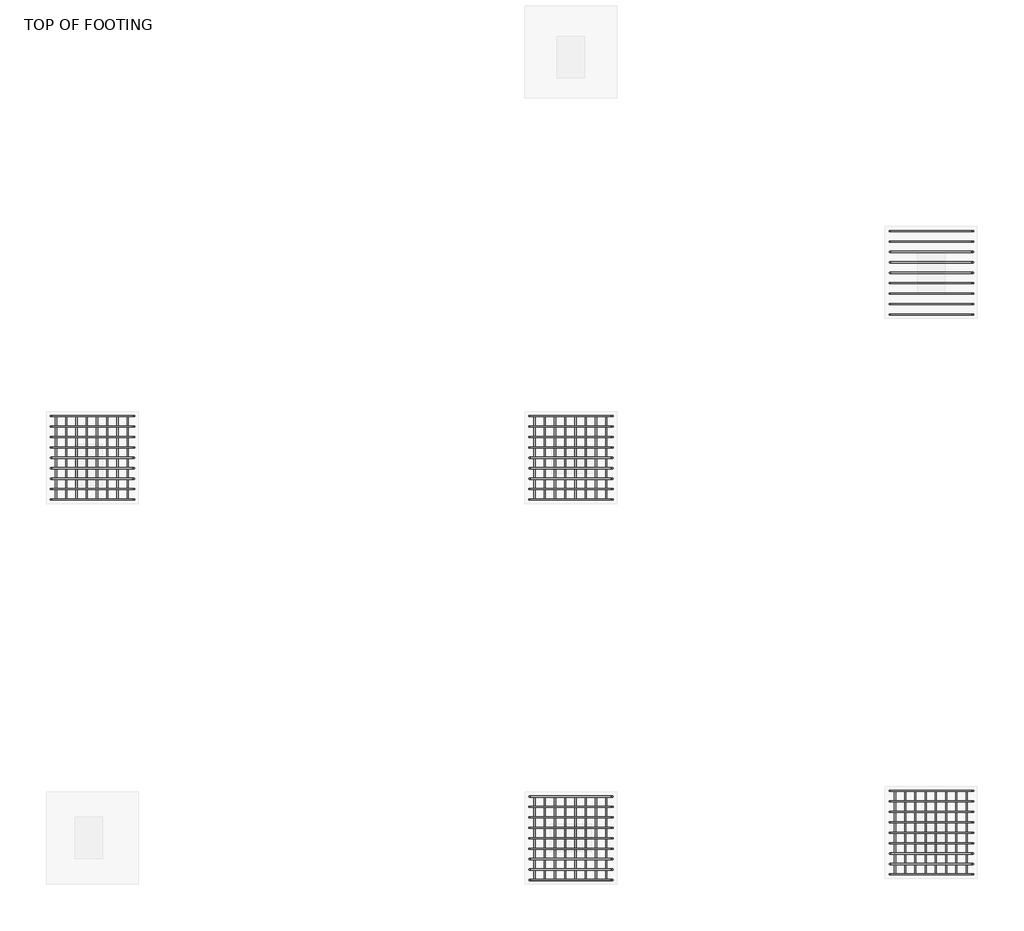
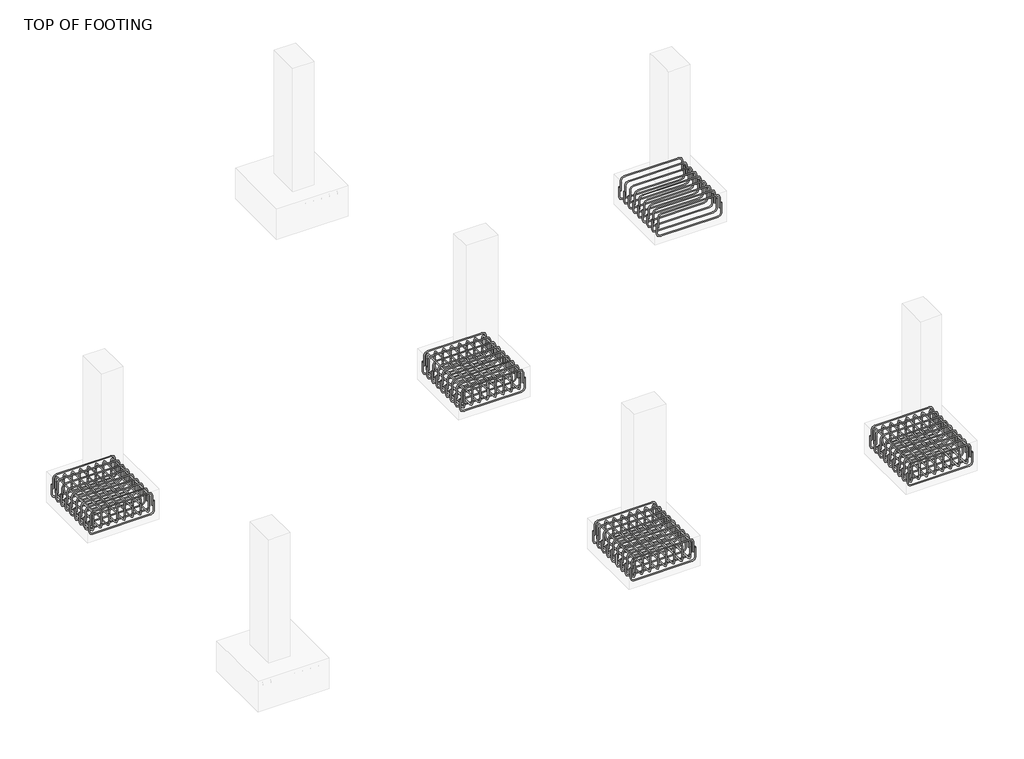
# One storey, part 11 of 20: 18 reinforcing bars.
"""IFC4 building model written with IfcOpenShell, lengths in millimetres."""

from ifc_helpers import new_model, si_unit, point, frame, origin, place, context, project, spatial, polyline, circle_curve, trimmed, segment, composite_curve, source, transform, mapped, element, save
from ifc_brep_helpers import swept_disk

model = new_model("IFC4")

# Units and contexts
model_context = context("Model", 3, world=origin())
ifc_project = project(units=[si_unit("LENGTHUNIT", "METRE", prefix="MILLI")], contexts=[model_context])

# Site, building, storey
site = spatial("IfcSite", under=ifc_project)
building = spatial("IfcBuilding", under=site)
storey = spatial("IfcBuildingStorey", under=building, Name="TOP OF FOOTING", Elevation=-1828.8)

# Reinforcing bars
placement = place(None, origin())
reinforcing_bar_shape = source(origin(), model_context, "Body", "SolidModel", [
    swept_disk(composite_curve([segment(polyline([(-1368.1365686, 1614.8213929, -2006.6587682), (-1368.1365686, 1614.8213929, -2153.9587682)]), True, "CONTINUOUS"), segment(trimmed(circle_curve(frame((-1414.4865686, 1614.8213929, -2153.9587682), z_axis=(0.0, 1.0, 0.0), x_axis=(46.350000000000136, 0.0, 0.0)), 46.35), [point((-1368.1365686, 1614.8213929, -2153.9587682))], [point((-1414.4865686, 1614.8213929, -2200.3087682))], True, "CARTESIAN"), True, "CONTINUOUS"), segment(polyline([(-1414.4865686, 1614.8213929, -2200.3087682), (-2229.0865686, 1614.8213929, -2200.3087682)]), True, "CONTINUOUS"), segment(trimmed(circle_curve(frame((-2229.0865686, 1614.8213929, -2153.9587682), z_axis=(0.0, 1.0, 0.0), x_axis=(0.0, 0.0, -46.34999999999991)), 46.35), [point((-2229.0865686, 1614.8213929, -2200.3087682))], [point((-2275.4365686, 1614.8213929, -2153.9587682))], True, "CARTESIAN"), True, "CONTINUOUS"), segment(polyline([(-2275.4365686, 1614.8213929, -2153.9587682), (-2275.4365686, 1614.8213929, -2006.6587682)]), True, "CONTINUOUS")], self_intersect=False), 6.35),
])
element("IfcReinforcingBar", 1, at=placement, inside=storey, context=model_context, shape_type="MappedRepresentation", body=[
    mapped(reinforcing_bar_shape, transform((0.0, 0.0, 0.0), x_axis=(1.0, 0.0, 0.0), y_axis=(0.0, 1.0, 0.0), z_axis=(0.0, 0.0, 1.0))),
    mapped(reinforcing_bar_shape, transform((0.0, -113.4125, 0.0), x_axis=(1.0, 0.0, 0.0), y_axis=(0.0, 1.0, 0.0), z_axis=(0.0, 0.0, 1.0))),
    mapped(reinforcing_bar_shape, transform((0.0, -226.825, 0.0), x_axis=(1.0, 0.0, 0.0), y_axis=(0.0, 1.0, 0.0), z_axis=(0.0, 0.0, 1.0))),
    mapped(reinforcing_bar_shape, transform((0.0, -340.2375, 0.0), x_axis=(1.0, 0.0, 0.0), y_axis=(0.0, 1.0, 0.0), z_axis=(0.0, 0.0, 1.0))),
    mapped(reinforcing_bar_shape, transform((0.0, -453.65, 0.0), x_axis=(1.0, 0.0, 0.0), y_axis=(0.0, 1.0, 0.0), z_axis=(0.0, 0.0, 1.0))),
    mapped(reinforcing_bar_shape, transform((0.0, -567.0625, 0.0), x_axis=(1.0, 0.0, 0.0), y_axis=(0.0, 1.0, 0.0), z_axis=(0.0, 0.0, 1.0))),
    mapped(reinforcing_bar_shape, transform((0.0, -680.475, 0.0), x_axis=(1.0, 0.0, 0.0), y_axis=(0.0, 1.0, 0.0), z_axis=(0.0, 0.0, 1.0))),
    mapped(reinforcing_bar_shape, transform((0.0, -793.8875, 0.0), x_axis=(1.0, 0.0, 0.0), y_axis=(0.0, 1.0, 0.0), z_axis=(0.0, 0.0, 1.0))),
    mapped(reinforcing_bar_shape, transform((0.0, -907.3, 0.0), x_axis=(1.0, 0.0, 0.0), y_axis=(0.0, 1.0, 0.0), z_axis=(0.0, 0.0, 1.0))),
])
reinforcing_bar_2_shape = source(origin(), model_context, "Body", "SolidModel", [
    swept_disk(composite_curve([segment(polyline([(-2255.9624573, 1614.8213929, -2068.8), (-2255.9624573, 1614.8213929, -1921.5)]), True, "CONTINUOUS"), segment(trimmed(circle_curve(frame((-2209.6124573, 1614.8213929, -1921.5), z_axis=(0.0, 1.0, 0.0), x_axis=(-46.34999999999991, 0.0, 0.0)), 46.35), [point((-2255.9624573, 1614.8213929, -1921.5))], [point((-2209.6124573, 1614.8213929, -1875.15))], True, "CARTESIAN"), True, "CONTINUOUS"), segment(polyline([(-2209.6124573, 1614.8213929, -1875.15), (-1440.1490576, 1614.8213929, -1875.15)]), True, "CONTINUOUS"), segment(trimmed(circle_curve(frame((-1440.1490576, 1614.8213929, -1921.5), z_axis=(0.0, 1.0, 0.0), x_axis=(0.0, 0.0, 46.34999999999991)), 46.35), [point((-1440.1490576, 1614.8213929, -1875.15))], [point((-1393.7990576, 1614.8213929, -1921.5))], True, "CARTESIAN"), True, "CONTINUOUS"), segment(polyline([(-1393.7990576, 1614.8213929, -1921.5), (-1393.7990576, 1614.8213929, -2068.8)]), True, "CONTINUOUS")], self_intersect=False), 6.35),
])
element("IfcReinforcingBar", 2, at=placement, inside=storey, context=model_context, shape_type="MappedRepresentation", body=[
    mapped(reinforcing_bar_2_shape, transform((0.0, 0.0, 0.0), x_axis=(1.0, 0.0, 0.0), y_axis=(0.0, 1.0, 0.0), z_axis=(0.0, 0.0, 1.0))),
    mapped(reinforcing_bar_2_shape, transform((0.0, -113.4125, 0.0), x_axis=(1.0, 0.0, 0.0), y_axis=(0.0, 1.0, 0.0), z_axis=(0.0, 0.0, 1.0))),
    mapped(reinforcing_bar_2_shape, transform((0.0, -226.825, 0.0), x_axis=(1.0, 0.0, 0.0), y_axis=(0.0, 1.0, 0.0), z_axis=(0.0, 0.0, 1.0))),
    mapped(reinforcing_bar_2_shape, transform((0.0, -340.2375, 0.0), x_axis=(1.0, 0.0, 0.0), y_axis=(0.0, 1.0, 0.0), z_axis=(0.0, 0.0, 1.0))),
    mapped(reinforcing_bar_2_shape, transform((0.0, -453.65, 0.0), x_axis=(1.0, 0.0, 0.0), y_axis=(0.0, 1.0, 0.0), z_axis=(0.0, 0.0, 1.0))),
    mapped(reinforcing_bar_2_shape, transform((0.0, -567.0625, 0.0), x_axis=(1.0, 0.0, 0.0), y_axis=(0.0, 1.0, 0.0), z_axis=(0.0, 0.0, 1.0))),
    mapped(reinforcing_bar_2_shape, transform((0.0, -680.475, 0.0), x_axis=(1.0, 0.0, 0.0), y_axis=(0.0, 1.0, 0.0), z_axis=(0.0, 0.0, 1.0))),
    mapped(reinforcing_bar_2_shape, transform((0.0, -793.8875, 0.0), x_axis=(1.0, 0.0, 0.0), y_axis=(0.0, 1.0, 0.0), z_axis=(0.0, 0.0, 1.0))),
    mapped(reinforcing_bar_2_shape, transform((0.0, -907.3, 0.0), x_axis=(1.0, 0.0, 0.0), y_axis=(0.0, 1.0, 0.0), z_axis=(0.0, 0.0, 1.0))),
])
reinforcing_bar_3_shape = source(origin(), model_context, "Body", "SolidModel", [
    swept_disk(composite_curve([segment(polyline([(-1439.63353, 1614.8213929, -2086.1951968), (-1439.63353, 1614.8213929, -1938.8951968)]), True, "CONTINUOUS"), segment(trimmed(circle_curve(frame((-1439.63353, 1568.4713929, -1938.8951968), z_axis=(1.0, 0.0, 0.0), x_axis=(0.0, 46.350000000000136, 0.0)), 46.35), [point((-1439.63353, 1614.8213929, -1938.8951968))], [point((-1439.63353, 1568.4713929, -1892.5451968))], True, "CARTESIAN"), True, "CONTINUOUS"), segment(polyline([(-1439.63353, 1568.4713929, -1892.5451968), (-1439.63353, 753.8713929, -1892.5451968)]), True, "CONTINUOUS"), segment(trimmed(circle_curve(frame((-1439.63353, 753.8713929, -1938.8951968), z_axis=(1.0, 0.0, 0.0), x_axis=(0.0, 0.0, 46.34999999999991)), 46.35), [point((-1439.63353, 753.8713929, -1892.5451968))], [point((-1439.63353, 707.5213929, -1938.8951968))], True, "CARTESIAN"), True, "CONTINUOUS"), segment(polyline([(-1439.63353, 707.5213929, -1938.8951968), (-1439.63353, 707.5213929, -2086.1951968)]), True, "CONTINUOUS")], self_intersect=False), 6.35),
])
element("IfcReinforcingBar", 3, at=placement, inside=storey, context=model_context, shape_type="MappedRepresentation", body=[
    mapped(reinforcing_bar_3_shape, transform((0.0, 0.0, 0.0), x_axis=(1.0, 0.0, 0.0), y_axis=(0.0, 1.0, 0.0), z_axis=(0.0, 0.0, 1.0))),
    mapped(reinforcing_bar_3_shape, transform((-111.2862402, 0.0, 0.0), x_axis=(1.0, 0.0, 0.0), y_axis=(0.0, 1.0, 0.0), z_axis=(0.0, 0.0, 1.0))),
    mapped(reinforcing_bar_3_shape, transform((-222.5724804, 0.0, 0.0), x_axis=(1.0, 0.0, 0.0), y_axis=(0.0, 1.0, 0.0), z_axis=(0.0, 0.0, 1.0))),
    mapped(reinforcing_bar_3_shape, transform((-333.8587205, 0.0, 0.0), x_axis=(1.0, 0.0, 0.0), y_axis=(0.0, 1.0, 0.0), z_axis=(0.0, 0.0, 1.0))),
    mapped(reinforcing_bar_3_shape, transform((-445.1449607, 0.0, 0.0), x_axis=(1.0, 0.0, 0.0), y_axis=(0.0, 1.0, 0.0), z_axis=(0.0, 0.0, 1.0))),
    mapped(reinforcing_bar_3_shape, transform((-556.4312009, 0.0, 0.0), x_axis=(1.0, 0.0, 0.0), y_axis=(0.0, 1.0, 0.0), z_axis=(0.0, 0.0, 1.0))),
    mapped(reinforcing_bar_3_shape, transform((-667.7174411, 0.0, 0.0), x_axis=(1.0, 0.0, 0.0), y_axis=(0.0, 1.0, 0.0), z_axis=(0.0, 0.0, 1.0))),
    mapped(reinforcing_bar_3_shape, transform((-779.0036813, 0.0, 0.0), x_axis=(1.0, 0.0, 0.0), y_axis=(0.0, 1.0, 0.0), z_axis=(0.0, 0.0, 1.0))),
])
reinforcing_bar_4_shape = source(origin(), model_context, "Body", "SolidModel", [
    swept_disk(composite_curve([segment(polyline([(-2218.6372113, 1614.8213929, -1979.1645013), (-2218.6372113, 1614.8213929, -2126.4645013)]), True, "CONTINUOUS"), segment(trimmed(circle_curve(frame((-2218.6372113, 1568.4713929, -2126.4645013), z_axis=(-1.0, 0.0, 0.0), x_axis=(0.0, 46.350000000000136, 0.0)), 46.35), [point((-2218.6372113, 1614.8213929, -2126.4645013))], [point((-2218.6372113, 1568.4713929, -2172.8145013))], True, "CARTESIAN"), True, "CONTINUOUS"), segment(polyline([(-2218.6372113, 1568.4713929, -2172.8145013), (-2218.6372113, 753.8713929, -2172.8145013)]), True, "CONTINUOUS"), segment(trimmed(circle_curve(frame((-2218.6372113, 753.8713929, -2126.4645013), z_axis=(-1.0, 0.0, 0.0), x_axis=(0.0, 0.0, -46.34999999999991)), 46.35), [point((-2218.6372113, 753.8713929, -2172.8145013))], [point((-2218.6372113, 707.5213929, -2126.4645013))], True, "CARTESIAN"), True, "CONTINUOUS"), segment(polyline([(-2218.6372113, 707.5213929, -2126.4645013), (-2218.6372113, 707.5213929, -1979.1645013)]), True, "CONTINUOUS")], self_intersect=False), 6.35),
])
element("IfcReinforcingBar", 4, at=placement, inside=storey, context=model_context, shape_type="MappedRepresentation", body=[
    mapped(reinforcing_bar_4_shape, transform((0.0, 0.0, 0.0), x_axis=(1.0, 0.0, 0.0), y_axis=(0.0, 1.0, 0.0), z_axis=(0.0, 0.0, 1.0))),
    mapped(reinforcing_bar_4_shape, transform((111.2862402, 0.0, 0.0), x_axis=(1.0, 0.0, 0.0), y_axis=(0.0, 1.0, 0.0), z_axis=(0.0, 0.0, 1.0))),
    mapped(reinforcing_bar_4_shape, transform((222.5724804, 0.0, 0.0), x_axis=(1.0, 0.0, 0.0), y_axis=(0.0, 1.0, 0.0), z_axis=(0.0, 0.0, 1.0))),
    mapped(reinforcing_bar_4_shape, transform((333.8587205, 0.0, 0.0), x_axis=(1.0, 0.0, 0.0), y_axis=(0.0, 1.0, 0.0), z_axis=(0.0, 0.0, 1.0))),
    mapped(reinforcing_bar_4_shape, transform((445.1449607, 0.0, 0.0), x_axis=(1.0, 0.0, 0.0), y_axis=(0.0, 1.0, 0.0), z_axis=(0.0, 0.0, 1.0))),
    mapped(reinforcing_bar_4_shape, transform((556.4312009, 0.0, 0.0), x_axis=(1.0, 0.0, 0.0), y_axis=(0.0, 1.0, 0.0), z_axis=(0.0, 0.0, 1.0))),
    mapped(reinforcing_bar_4_shape, transform((667.7174411, 0.0, 0.0), x_axis=(1.0, 0.0, 0.0), y_axis=(0.0, 1.0, 0.0), z_axis=(0.0, 0.0, 1.0))),
    mapped(reinforcing_bar_4_shape, transform((779.0036813, 0.0, 0.0), x_axis=(1.0, 0.0, 0.0), y_axis=(0.0, 1.0, 0.0), z_axis=(0.0, 0.0, 1.0))),
])
reinforcing_bar_5_shape = source(origin(), model_context, "Body", "SolidModel", [
    swept_disk(composite_curve([segment(polyline([(-5285.1605653, 1554.8213929, -2006.6587682), (-5285.1605653, 1554.8213929, -2153.9587682)]), True, "CONTINUOUS"), segment(trimmed(circle_curve(frame((-5331.5105653, 1554.8213929, -2153.9587682), z_axis=(0.0, 1.0, 0.0), x_axis=(46.350000000000364, 0.0, 0.0)), 46.35), [point((-5285.1605653, 1554.8213929, -2153.9587682))], [point((-5331.5105653, 1554.8213929, -2200.3087682))], True, "CARTESIAN"), True, "CONTINUOUS"), segment(polyline([(-5331.5105653, 1554.8213929, -2200.3087682), (-6146.1105653, 1554.8213929, -2200.3087682)]), True, "CONTINUOUS"), segment(trimmed(circle_curve(frame((-6146.1105653, 1554.8213929, -2153.9587682), z_axis=(0.0, 1.0, 0.0), x_axis=(0.0, 0.0, -46.34999999999991)), 46.35), [point((-6146.1105653, 1554.8213929, -2200.3087682))], [point((-6192.4605653, 1554.8213929, -2153.9587682))], True, "CARTESIAN"), True, "CONTINUOUS"), segment(polyline([(-6192.4605653, 1554.8213929, -2153.9587682), (-6192.4605653, 1554.8213929, -2006.6587682)]), True, "CONTINUOUS")], self_intersect=False), 6.35),
])
element("IfcReinforcingBar", 5, at=placement, inside=storey, context=model_context, shape_type="MappedRepresentation", body=[
    mapped(reinforcing_bar_5_shape, transform((0.0, 0.0, 0.0), x_axis=(1.0, 0.0, 0.0), y_axis=(0.0, 1.0, 0.0), z_axis=(0.0, 0.0, 1.0))),
    mapped(reinforcing_bar_5_shape, transform((0.0, -113.4125, 0.0), x_axis=(1.0, 0.0, 0.0), y_axis=(0.0, 1.0, 0.0), z_axis=(0.0, 0.0, 1.0))),
    mapped(reinforcing_bar_5_shape, transform((0.0, -226.825, 0.0), x_axis=(1.0, 0.0, 0.0), y_axis=(0.0, 1.0, 0.0), z_axis=(0.0, 0.0, 1.0))),
    mapped(reinforcing_bar_5_shape, transform((0.0, -340.2375, 0.0), x_axis=(1.0, 0.0, 0.0), y_axis=(0.0, 1.0, 0.0), z_axis=(0.0, 0.0, 1.0))),
    mapped(reinforcing_bar_5_shape, transform((0.0, -453.65, 0.0), x_axis=(1.0, 0.0, 0.0), y_axis=(0.0, 1.0, 0.0), z_axis=(0.0, 0.0, 1.0))),
    mapped(reinforcing_bar_5_shape, transform((0.0, -567.0625, 0.0), x_axis=(1.0, 0.0, 0.0), y_axis=(0.0, 1.0, 0.0), z_axis=(0.0, 0.0, 1.0))),
    mapped(reinforcing_bar_5_shape, transform((0.0, -680.475, 0.0), x_axis=(1.0, 0.0, 0.0), y_axis=(0.0, 1.0, 0.0), z_axis=(0.0, 0.0, 1.0))),
    mapped(reinforcing_bar_5_shape, transform((0.0, -793.8875, 0.0), x_axis=(1.0, 0.0, 0.0), y_axis=(0.0, 1.0, 0.0), z_axis=(0.0, 0.0, 1.0))),
    mapped(reinforcing_bar_5_shape, transform((0.0, -907.3, 0.0), x_axis=(1.0, 0.0, 0.0), y_axis=(0.0, 1.0, 0.0), z_axis=(0.0, 0.0, 1.0))),
])
reinforcing_bar_6_shape = source(origin(), model_context, "Body", "SolidModel", [
    swept_disk(composite_curve([segment(polyline([(-6172.986454, 1554.8213929, -2068.8), (-6172.986454, 1554.8213929, -1921.5)]), True, "CONTINUOUS"), segment(trimmed(circle_curve(frame((-6126.636454, 1554.8213929, -1921.5), z_axis=(0.0, 1.0, 0.0), x_axis=(-46.349999999999454, 0.0, 0.0)), 46.35), [point((-6172.986454, 1554.8213929, -1921.5))], [point((-6126.636454, 1554.8213929, -1875.15))], True, "CARTESIAN"), True, "CONTINUOUS"), segment(polyline([(-6126.636454, 1554.8213929, -1875.15), (-5357.1730543, 1554.8213929, -1875.15)]), True, "CONTINUOUS"), segment(trimmed(circle_curve(frame((-5357.1730543, 1554.8213929, -1921.5), z_axis=(0.0, 1.0, 0.0), x_axis=(0.0, 0.0, 46.34999999999991)), 46.35), [point((-5357.1730543, 1554.8213929, -1875.15))], [point((-5310.8230543, 1554.8213929, -1921.5))], True, "CARTESIAN"), True, "CONTINUOUS"), segment(polyline([(-5310.8230543, 1554.8213929, -1921.5), (-5310.8230543, 1554.8213929, -2068.8)]), True, "CONTINUOUS")], self_intersect=False), 6.35),
])
element("IfcReinforcingBar", 6, at=placement, inside=storey, context=model_context, shape_type="MappedRepresentation", body=[
    mapped(reinforcing_bar_6_shape, transform((0.0, 0.0, 0.0), x_axis=(1.0, 0.0, 0.0), y_axis=(0.0, 1.0, 0.0), z_axis=(0.0, 0.0, 1.0))),
    mapped(reinforcing_bar_6_shape, transform((0.0, -113.4125, 0.0), x_axis=(1.0, 0.0, 0.0), y_axis=(0.0, 1.0, 0.0), z_axis=(0.0, 0.0, 1.0))),
    mapped(reinforcing_bar_6_shape, transform((0.0, -226.825, 0.0), x_axis=(1.0, 0.0, 0.0), y_axis=(0.0, 1.0, 0.0), z_axis=(0.0, 0.0, 1.0))),
    mapped(reinforcing_bar_6_shape, transform((0.0, -340.2375, 0.0), x_axis=(1.0, 0.0, 0.0), y_axis=(0.0, 1.0, 0.0), z_axis=(0.0, 0.0, 1.0))),
    mapped(reinforcing_bar_6_shape, transform((0.0, -453.65, 0.0), x_axis=(1.0, 0.0, 0.0), y_axis=(0.0, 1.0, 0.0), z_axis=(0.0, 0.0, 1.0))),
    mapped(reinforcing_bar_6_shape, transform((0.0, -567.0625, 0.0), x_axis=(1.0, 0.0, 0.0), y_axis=(0.0, 1.0, 0.0), z_axis=(0.0, 0.0, 1.0))),
    mapped(reinforcing_bar_6_shape, transform((0.0, -680.475, 0.0), x_axis=(1.0, 0.0, 0.0), y_axis=(0.0, 1.0, 0.0), z_axis=(0.0, 0.0, 1.0))),
    mapped(reinforcing_bar_6_shape, transform((0.0, -793.8875, 0.0), x_axis=(1.0, 0.0, 0.0), y_axis=(0.0, 1.0, 0.0), z_axis=(0.0, 0.0, 1.0))),
    mapped(reinforcing_bar_6_shape, transform((0.0, -907.3, 0.0), x_axis=(1.0, 0.0, 0.0), y_axis=(0.0, 1.0, 0.0), z_axis=(0.0, 0.0, 1.0))),
])
reinforcing_bar_7_shape = source(origin(), model_context, "Body", "SolidModel", [
    swept_disk(composite_curve([segment(polyline([(-5356.6575267, 1554.8213929, -2086.1951968), (-5356.6575267, 1554.8213929, -1938.8951968)]), True, "CONTINUOUS"), segment(trimmed(circle_curve(frame((-5356.6575267, 1508.4713929, -1938.8951968), z_axis=(1.0, 0.0, 0.0), x_axis=(0.0, 46.350000000000136, 0.0)), 46.35), [point((-5356.6575267, 1554.8213929, -1938.8951968))], [point((-5356.6575267, 1508.4713929, -1892.5451968))], True, "CARTESIAN"), True, "CONTINUOUS"), segment(polyline([(-5356.6575267, 1508.4713929, -1892.5451968), (-5356.6575267, 693.8713929, -1892.5451968)]), True, "CONTINUOUS"), segment(trimmed(circle_curve(frame((-5356.6575267, 693.8713929, -1938.8951968), z_axis=(1.0, 0.0, 0.0), x_axis=(0.0, 0.0, 46.34999999999991)), 46.35), [point((-5356.6575267, 693.8713929, -1892.5451968))], [point((-5356.6575267, 647.5213929, -1938.8951968))], True, "CARTESIAN"), True, "CONTINUOUS"), segment(polyline([(-5356.6575267, 647.5213929, -1938.8951968), (-5356.6575267, 647.5213929, -2086.1951968)]), True, "CONTINUOUS")], self_intersect=False), 6.35),
])
element("IfcReinforcingBar", 7, at=placement, inside=storey, context=model_context, shape_type="MappedRepresentation", body=[
    mapped(reinforcing_bar_7_shape, transform((0.0, 0.0, 0.0), x_axis=(1.0, 0.0, 0.0), y_axis=(0.0, 1.0, 0.0), z_axis=(0.0, 0.0, 1.0))),
    mapped(reinforcing_bar_7_shape, transform((-111.2862402, 0.0, 0.0), x_axis=(1.0, 0.0, 0.0), y_axis=(0.0, 1.0, 0.0), z_axis=(0.0, 0.0, 1.0))),
    mapped(reinforcing_bar_7_shape, transform((-222.5724804, 0.0, 0.0), x_axis=(1.0, 0.0, 0.0), y_axis=(0.0, 1.0, 0.0), z_axis=(0.0, 0.0, 1.0))),
    mapped(reinforcing_bar_7_shape, transform((-333.8587205, 0.0, 0.0), x_axis=(1.0, 0.0, 0.0), y_axis=(0.0, 1.0, 0.0), z_axis=(0.0, 0.0, 1.0))),
    mapped(reinforcing_bar_7_shape, transform((-445.1449607, 0.0, 0.0), x_axis=(1.0, 0.0, 0.0), y_axis=(0.0, 1.0, 0.0), z_axis=(0.0, 0.0, 1.0))),
    mapped(reinforcing_bar_7_shape, transform((-556.4312009, 0.0, 0.0), x_axis=(1.0, 0.0, 0.0), y_axis=(0.0, 1.0, 0.0), z_axis=(0.0, 0.0, 1.0))),
    mapped(reinforcing_bar_7_shape, transform((-667.7174411, 0.0, 0.0), x_axis=(1.0, 0.0, 0.0), y_axis=(0.0, 1.0, 0.0), z_axis=(0.0, 0.0, 1.0))),
    mapped(reinforcing_bar_7_shape, transform((-779.0036813, 0.0, 0.0), x_axis=(1.0, 0.0, 0.0), y_axis=(0.0, 1.0, 0.0), z_axis=(0.0, 0.0, 1.0))),
])
reinforcing_bar_8_shape = source(origin(), model_context, "Body", "SolidModel", [
    swept_disk(composite_curve([segment(polyline([(-6135.661208, 1554.8213929, -1979.1645013), (-6135.661208, 1554.8213929, -2126.4645013)]), True, "CONTINUOUS"), segment(trimmed(circle_curve(frame((-6135.661208, 1508.4713929, -2126.4645013), z_axis=(-1.0, 0.0, 0.0), x_axis=(0.0, 46.350000000000136, 0.0)), 46.35), [point((-6135.661208, 1554.8213929, -2126.4645013))], [point((-6135.661208, 1508.4713929, -2172.8145013))], True, "CARTESIAN"), True, "CONTINUOUS"), segment(polyline([(-6135.661208, 1508.4713929, -2172.8145013), (-6135.661208, 693.8713929, -2172.8145013)]), True, "CONTINUOUS"), segment(trimmed(circle_curve(frame((-6135.661208, 693.8713929, -2126.4645013), z_axis=(-1.0, 0.0, 0.0), x_axis=(0.0, 0.0, -46.34999999999991)), 46.35), [point((-6135.661208, 693.8713929, -2172.8145013))], [point((-6135.661208, 647.5213929, -2126.4645013))], True, "CARTESIAN"), True, "CONTINUOUS"), segment(polyline([(-6135.661208, 647.5213929, -2126.4645013), (-6135.661208, 647.5213929, -1979.1645013)]), True, "CONTINUOUS")], self_intersect=False), 6.35),
])
element("IfcReinforcingBar", 8, at=placement, inside=storey, context=model_context, shape_type="MappedRepresentation", body=[
    mapped(reinforcing_bar_8_shape, transform((0.0, 0.0, 0.0), x_axis=(1.0, 0.0, 0.0), y_axis=(0.0, 1.0, 0.0), z_axis=(0.0, 0.0, 1.0))),
    mapped(reinforcing_bar_8_shape, transform((111.2862402, 0.0, 0.0), x_axis=(1.0, 0.0, 0.0), y_axis=(0.0, 1.0, 0.0), z_axis=(0.0, 0.0, 1.0))),
    mapped(reinforcing_bar_8_shape, transform((222.5724804, 0.0, 0.0), x_axis=(1.0, 0.0, 0.0), y_axis=(0.0, 1.0, 0.0), z_axis=(0.0, 0.0, 1.0))),
    mapped(reinforcing_bar_8_shape, transform((333.8587205, 0.0, 0.0), x_axis=(1.0, 0.0, 0.0), y_axis=(0.0, 1.0, 0.0), z_axis=(0.0, 0.0, 1.0))),
    mapped(reinforcing_bar_8_shape, transform((445.1449607, 0.0, 0.0), x_axis=(1.0, 0.0, 0.0), y_axis=(0.0, 1.0, 0.0), z_axis=(0.0, 0.0, 1.0))),
    mapped(reinforcing_bar_8_shape, transform((556.4312009, 0.0, 0.0), x_axis=(1.0, 0.0, 0.0), y_axis=(0.0, 1.0, 0.0), z_axis=(0.0, 0.0, 1.0))),
    mapped(reinforcing_bar_8_shape, transform((667.7174411, 0.0, 0.0), x_axis=(1.0, 0.0, 0.0), y_axis=(0.0, 1.0, 0.0), z_axis=(0.0, 0.0, 1.0))),
    mapped(reinforcing_bar_8_shape, transform((779.0036813, 0.0, 0.0), x_axis=(1.0, 0.0, 0.0), y_axis=(0.0, 1.0, 0.0), z_axis=(0.0, 0.0, 1.0))),
])
reinforcing_bar_9_shape = source(origin(), model_context, "Body", "SolidModel", [
    swept_disk(composite_curve([segment(polyline([(-5285.1605653, 5691.2557249, -2006.6587682), (-5285.1605653, 5691.2557249, -2153.9587682)]), True, "CONTINUOUS"), segment(trimmed(circle_curve(frame((-5331.5105653, 5691.2557249, -2153.9587682), z_axis=(0.0, 1.0, 0.0), x_axis=(46.350000000000364, 0.0, 0.0)), 46.35), [point((-5285.1605653, 5691.2557249, -2153.9587682))], [point((-5331.5105653, 5691.2557249, -2200.3087682))], True, "CARTESIAN"), True, "CONTINUOUS"), segment(polyline([(-5331.5105653, 5691.2557249, -2200.3087682), (-6146.1105653, 5691.2557249, -2200.3087682)]), True, "CONTINUOUS"), segment(trimmed(circle_curve(frame((-6146.1105653, 5691.2557249, -2153.9587682), z_axis=(0.0, 1.0, 0.0), x_axis=(0.0, 0.0, -46.34999999999991)), 46.35), [point((-6146.1105653, 5691.2557249, -2200.3087682))], [point((-6192.4605653, 5691.2557249, -2153.9587682))], True, "CARTESIAN"), True, "CONTINUOUS"), segment(polyline([(-6192.4605653, 5691.2557249, -2153.9587682), (-6192.4605653, 5691.2557249, -2006.6587682)]), True, "CONTINUOUS")], self_intersect=False), 6.35),
])
element("IfcReinforcingBar", 9, at=placement, inside=storey, context=model_context, shape_type="MappedRepresentation", body=[
    mapped(reinforcing_bar_9_shape, transform((0.0, 0.0, 0.0), x_axis=(1.0, 0.0, 0.0), y_axis=(0.0, 1.0, 0.0), z_axis=(0.0, 0.0, 1.0))),
    mapped(reinforcing_bar_9_shape, transform((0.0, -113.4125, 0.0), x_axis=(1.0, 0.0, 0.0), y_axis=(0.0, 1.0, 0.0), z_axis=(0.0, 0.0, 1.0))),
    mapped(reinforcing_bar_9_shape, transform((0.0, -226.825, 0.0), x_axis=(1.0, 0.0, 0.0), y_axis=(0.0, 1.0, 0.0), z_axis=(0.0, 0.0, 1.0))),
    mapped(reinforcing_bar_9_shape, transform((0.0, -340.2375, 0.0), x_axis=(1.0, 0.0, 0.0), y_axis=(0.0, 1.0, 0.0), z_axis=(0.0, 0.0, 1.0))),
    mapped(reinforcing_bar_9_shape, transform((0.0, -453.65, 0.0), x_axis=(1.0, 0.0, 0.0), y_axis=(0.0, 1.0, 0.0), z_axis=(0.0, 0.0, 1.0))),
    mapped(reinforcing_bar_9_shape, transform((0.0, -567.0625, 0.0), x_axis=(1.0, 0.0, 0.0), y_axis=(0.0, 1.0, 0.0), z_axis=(0.0, 0.0, 1.0))),
    mapped(reinforcing_bar_9_shape, transform((0.0, -680.475, 0.0), x_axis=(1.0, 0.0, 0.0), y_axis=(0.0, 1.0, 0.0), z_axis=(0.0, 0.0, 1.0))),
    mapped(reinforcing_bar_9_shape, transform((0.0, -793.8875, 0.0), x_axis=(1.0, 0.0, 0.0), y_axis=(0.0, 1.0, 0.0), z_axis=(0.0, 0.0, 1.0))),
    mapped(reinforcing_bar_9_shape, transform((0.0, -907.3, 0.0), x_axis=(1.0, 0.0, 0.0), y_axis=(0.0, 1.0, 0.0), z_axis=(0.0, 0.0, 1.0))),
])
reinforcing_bar_10_shape = source(origin(), model_context, "Body", "SolidModel", [
    swept_disk(composite_curve([segment(polyline([(-6172.986454, 5691.2557249, -2068.8), (-6172.986454, 5691.2557249, -1921.5)]), True, "CONTINUOUS"), segment(trimmed(circle_curve(frame((-6126.636454, 5691.2557249, -1921.5), z_axis=(0.0, 1.0, 0.0), x_axis=(-46.349999999999454, 0.0, 0.0)), 46.35), [point((-6172.986454, 5691.2557249, -1921.5))], [point((-6126.636454, 5691.2557249, -1875.15))], True, "CARTESIAN"), True, "CONTINUOUS"), segment(polyline([(-6126.636454, 5691.2557249, -1875.15), (-5357.1730543, 5691.2557249, -1875.15)]), True, "CONTINUOUS"), segment(trimmed(circle_curve(frame((-5357.1730543, 5691.2557249, -1921.5), z_axis=(0.0, 1.0, 0.0), x_axis=(0.0, 0.0, 46.34999999999991)), 46.35), [point((-5357.1730543, 5691.2557249, -1875.15))], [point((-5310.8230543, 5691.2557249, -1921.5))], True, "CARTESIAN"), True, "CONTINUOUS"), segment(polyline([(-5310.8230543, 5691.2557249, -1921.5), (-5310.8230543, 5691.2557249, -2068.8)]), True, "CONTINUOUS")], self_intersect=False), 6.35),
])
element("IfcReinforcingBar", 10, at=placement, inside=storey, context=model_context, shape_type="MappedRepresentation", body=[
    mapped(reinforcing_bar_10_shape, transform((0.0, 0.0, 0.0), x_axis=(1.0, 0.0, 0.0), y_axis=(0.0, 1.0, 0.0), z_axis=(0.0, 0.0, 1.0))),
    mapped(reinforcing_bar_10_shape, transform((0.0, -113.4125, 0.0), x_axis=(1.0, 0.0, 0.0), y_axis=(0.0, 1.0, 0.0), z_axis=(0.0, 0.0, 1.0))),
    mapped(reinforcing_bar_10_shape, transform((0.0, -226.825, 0.0), x_axis=(1.0, 0.0, 0.0), y_axis=(0.0, 1.0, 0.0), z_axis=(0.0, 0.0, 1.0))),
    mapped(reinforcing_bar_10_shape, transform((0.0, -340.2375, 0.0), x_axis=(1.0, 0.0, 0.0), y_axis=(0.0, 1.0, 0.0), z_axis=(0.0, 0.0, 1.0))),
    mapped(reinforcing_bar_10_shape, transform((0.0, -453.65, 0.0), x_axis=(1.0, 0.0, 0.0), y_axis=(0.0, 1.0, 0.0), z_axis=(0.0, 0.0, 1.0))),
    mapped(reinforcing_bar_10_shape, transform((0.0, -567.0625, 0.0), x_axis=(1.0, 0.0, 0.0), y_axis=(0.0, 1.0, 0.0), z_axis=(0.0, 0.0, 1.0))),
    mapped(reinforcing_bar_10_shape, transform((0.0, -680.475, 0.0), x_axis=(1.0, 0.0, 0.0), y_axis=(0.0, 1.0, 0.0), z_axis=(0.0, 0.0, 1.0))),
    mapped(reinforcing_bar_10_shape, transform((0.0, -793.8875, 0.0), x_axis=(1.0, 0.0, 0.0), y_axis=(0.0, 1.0, 0.0), z_axis=(0.0, 0.0, 1.0))),
    mapped(reinforcing_bar_10_shape, transform((0.0, -907.3, 0.0), x_axis=(1.0, 0.0, 0.0), y_axis=(0.0, 1.0, 0.0), z_axis=(0.0, 0.0, 1.0))),
])
reinforcing_bar_11_shape = source(origin(), model_context, "Body", "SolidModel", [
    swept_disk(composite_curve([segment(polyline([(-5356.6575267, 5691.2557249, -2086.1951968), (-5356.6575267, 5691.2557249, -1938.8951968)]), True, "CONTINUOUS"), segment(trimmed(circle_curve(frame((-5356.6575267, 5644.9057249, -1938.8951968), z_axis=(1.0, 0.0, 0.0), x_axis=(0.0, 46.350000000000364, 0.0)), 46.35), [point((-5356.6575267, 5691.2557249, -1938.8951968))], [point((-5356.6575267, 5644.9057249, -1892.5451968))], True, "CARTESIAN"), True, "CONTINUOUS"), segment(polyline([(-5356.6575267, 5644.9057249, -1892.5451968), (-5356.6575267, 4830.3057249, -1892.5451968)]), True, "CONTINUOUS"), segment(trimmed(circle_curve(frame((-5356.6575267, 4830.3057249, -1938.8951968), z_axis=(1.0, 0.0, 0.0), x_axis=(0.0, 0.0, 46.34999999999991)), 46.35), [point((-5356.6575267, 4830.3057249, -1892.5451968))], [point((-5356.6575267, 4783.9557249, -1938.8951968))], True, "CARTESIAN"), True, "CONTINUOUS"), segment(polyline([(-5356.6575267, 4783.9557249, -1938.8951968), (-5356.6575267, 4783.9557249, -2086.1951968)]), True, "CONTINUOUS")], self_intersect=False), 6.35),
])
element("IfcReinforcingBar", 11, at=placement, inside=storey, context=model_context, shape_type="MappedRepresentation", body=[
    mapped(reinforcing_bar_11_shape, transform((0.0, 0.0, 0.0), x_axis=(1.0, 0.0, 0.0), y_axis=(0.0, 1.0, 0.0), z_axis=(0.0, 0.0, 1.0))),
    mapped(reinforcing_bar_11_shape, transform((-111.2862402, 0.0, 0.0), x_axis=(1.0, 0.0, 0.0), y_axis=(0.0, 1.0, 0.0), z_axis=(0.0, 0.0, 1.0))),
    mapped(reinforcing_bar_11_shape, transform((-222.5724804, 0.0, 0.0), x_axis=(1.0, 0.0, 0.0), y_axis=(0.0, 1.0, 0.0), z_axis=(0.0, 0.0, 1.0))),
    mapped(reinforcing_bar_11_shape, transform((-333.8587205, 0.0, 0.0), x_axis=(1.0, 0.0, 0.0), y_axis=(0.0, 1.0, 0.0), z_axis=(0.0, 0.0, 1.0))),
    mapped(reinforcing_bar_11_shape, transform((-445.1449607, 0.0, 0.0), x_axis=(1.0, 0.0, 0.0), y_axis=(0.0, 1.0, 0.0), z_axis=(0.0, 0.0, 1.0))),
    mapped(reinforcing_bar_11_shape, transform((-556.4312009, 0.0, 0.0), x_axis=(1.0, 0.0, 0.0), y_axis=(0.0, 1.0, 0.0), z_axis=(0.0, 0.0, 1.0))),
    mapped(reinforcing_bar_11_shape, transform((-667.7174411, 0.0, 0.0), x_axis=(1.0, 0.0, 0.0), y_axis=(0.0, 1.0, 0.0), z_axis=(0.0, 0.0, 1.0))),
    mapped(reinforcing_bar_11_shape, transform((-779.0036813, 0.0, 0.0), x_axis=(1.0, 0.0, 0.0), y_axis=(0.0, 1.0, 0.0), z_axis=(0.0, 0.0, 1.0))),
])
reinforcing_bar_12_shape = source(origin(), model_context, "Body", "SolidModel", [
    swept_disk(composite_curve([segment(polyline([(-6135.661208, 5691.2557249, -1979.1645013), (-6135.661208, 5691.2557249, -2126.4645013)]), True, "CONTINUOUS"), segment(trimmed(circle_curve(frame((-6135.661208, 5644.9057249, -2126.4645013), z_axis=(-1.0, 0.0, 0.0), x_axis=(0.0, 46.350000000000364, 0.0)), 46.35), [point((-6135.661208, 5691.2557249, -2126.4645013))], [point((-6135.661208, 5644.9057249, -2172.8145013))], True, "CARTESIAN"), True, "CONTINUOUS"), segment(polyline([(-6135.661208, 5644.9057249, -2172.8145013), (-6135.661208, 4830.3057249, -2172.8145013)]), True, "CONTINUOUS"), segment(trimmed(circle_curve(frame((-6135.661208, 4830.3057249, -2126.4645013), z_axis=(-1.0, 0.0, 0.0), x_axis=(0.0, 0.0, -46.34999999999991)), 46.35), [point((-6135.661208, 4830.3057249, -2172.8145013))], [point((-6135.661208, 4783.9557249, -2126.4645013))], True, "CARTESIAN"), True, "CONTINUOUS"), segment(polyline([(-6135.661208, 4783.9557249, -2126.4645013), (-6135.661208, 4783.9557249, -1979.1645013)]), True, "CONTINUOUS")], self_intersect=False), 6.35),
])
element("IfcReinforcingBar", 12, at=placement, inside=storey, context=model_context, shape_type="MappedRepresentation", body=[
    mapped(reinforcing_bar_12_shape, transform((0.0, 0.0, 0.0), x_axis=(1.0, 0.0, 0.0), y_axis=(0.0, 1.0, 0.0), z_axis=(0.0, 0.0, 1.0))),
    mapped(reinforcing_bar_12_shape, transform((111.2862402, 0.0, 0.0), x_axis=(1.0, 0.0, 0.0), y_axis=(0.0, 1.0, 0.0), z_axis=(0.0, 0.0, 1.0))),
    mapped(reinforcing_bar_12_shape, transform((222.5724804, 0.0, 0.0), x_axis=(1.0, 0.0, 0.0), y_axis=(0.0, 1.0, 0.0), z_axis=(0.0, 0.0, 1.0))),
    mapped(reinforcing_bar_12_shape, transform((333.8587205, 0.0, 0.0), x_axis=(1.0, 0.0, 0.0), y_axis=(0.0, 1.0, 0.0), z_axis=(0.0, 0.0, 1.0))),
    mapped(reinforcing_bar_12_shape, transform((445.1449607, 0.0, 0.0), x_axis=(1.0, 0.0, 0.0), y_axis=(0.0, 1.0, 0.0), z_axis=(0.0, 0.0, 1.0))),
    mapped(reinforcing_bar_12_shape, transform((556.4312009, 0.0, 0.0), x_axis=(1.0, 0.0, 0.0), y_axis=(0.0, 1.0, 0.0), z_axis=(0.0, 0.0, 1.0))),
    mapped(reinforcing_bar_12_shape, transform((667.7174411, 0.0, 0.0), x_axis=(1.0, 0.0, 0.0), y_axis=(0.0, 1.0, 0.0), z_axis=(0.0, 0.0, 1.0))),
    mapped(reinforcing_bar_12_shape, transform((779.0036813, 0.0, 0.0), x_axis=(1.0, 0.0, 0.0), y_axis=(0.0, 1.0, 0.0), z_axis=(0.0, 0.0, 1.0))),
])
reinforcing_bar_13_shape = source(origin(), model_context, "Body", "SolidModel", [
    swept_disk(composite_curve([segment(polyline([(-1368.1365686, 7703.3576276, -2006.6587682), (-1368.1365686, 7703.3576276, -2153.9587682)]), True, "CONTINUOUS"), segment(trimmed(circle_curve(frame((-1414.4865686, 7703.3576276, -2153.9587682), z_axis=(0.0, 1.0, 0.0), x_axis=(46.350000000000136, 0.0, 0.0)), 46.35), [point((-1368.1365686, 7703.3576276, -2153.9587682))], [point((-1414.4865686, 7703.3576276, -2200.3087682))], True, "CARTESIAN"), True, "CONTINUOUS"), segment(polyline([(-1414.4865686, 7703.3576276, -2200.3087682), (-2229.0865686, 7703.3576276, -2200.3087682)]), True, "CONTINUOUS"), segment(trimmed(circle_curve(frame((-2229.0865686, 7703.3576276, -2153.9587682), z_axis=(0.0, 1.0, 0.0), x_axis=(0.0, 0.0, -46.34999999999991)), 46.35), [point((-2229.0865686, 7703.3576276, -2200.3087682))], [point((-2275.4365686, 7703.3576276, -2153.9587682))], True, "CARTESIAN"), True, "CONTINUOUS"), segment(polyline([(-2275.4365686, 7703.3576276, -2153.9587682), (-2275.4365686, 7703.3576276, -2006.6587682)]), True, "CONTINUOUS")], self_intersect=False), 6.35),
])
element("IfcReinforcingBar", 13, at=placement, inside=storey, context=model_context, shape_type="MappedRepresentation", body=[
    mapped(reinforcing_bar_13_shape, transform((0.0, 0.0, 0.0), x_axis=(1.0, 0.0, 0.0), y_axis=(0.0, 1.0, 0.0), z_axis=(0.0, 0.0, 1.0))),
    mapped(reinforcing_bar_13_shape, transform((0.0, -113.4125, 0.0), x_axis=(1.0, 0.0, 0.0), y_axis=(0.0, 1.0, 0.0), z_axis=(0.0, 0.0, 1.0))),
    mapped(reinforcing_bar_13_shape, transform((0.0, -226.825, 0.0), x_axis=(1.0, 0.0, 0.0), y_axis=(0.0, 1.0, 0.0), z_axis=(0.0, 0.0, 1.0))),
    mapped(reinforcing_bar_13_shape, transform((0.0, -340.2375, 0.0), x_axis=(1.0, 0.0, 0.0), y_axis=(0.0, 1.0, 0.0), z_axis=(0.0, 0.0, 1.0))),
    mapped(reinforcing_bar_13_shape, transform((0.0, -453.65, 0.0), x_axis=(1.0, 0.0, 0.0), y_axis=(0.0, 1.0, 0.0), z_axis=(0.0, 0.0, 1.0))),
    mapped(reinforcing_bar_13_shape, transform((0.0, -567.0625, 0.0), x_axis=(1.0, 0.0, 0.0), y_axis=(0.0, 1.0, 0.0), z_axis=(0.0, 0.0, 1.0))),
    mapped(reinforcing_bar_13_shape, transform((0.0, -680.475, 0.0), x_axis=(1.0, 0.0, 0.0), y_axis=(0.0, 1.0, 0.0), z_axis=(0.0, 0.0, 1.0))),
    mapped(reinforcing_bar_13_shape, transform((0.0, -793.8875, 0.0), x_axis=(1.0, 0.0, 0.0), y_axis=(0.0, 1.0, 0.0), z_axis=(0.0, 0.0, 1.0))),
    mapped(reinforcing_bar_13_shape, transform((0.0, -907.3, 0.0), x_axis=(1.0, 0.0, 0.0), y_axis=(0.0, 1.0, 0.0), z_axis=(0.0, 0.0, 1.0))),
])
reinforcing_bar_14_shape = source(origin(), model_context, "Body", "SolidModel", [
    swept_disk(composite_curve([segment(polyline([(-2255.9624573, 7703.3576276, -2068.8), (-2255.9624573, 7703.3576276, -1921.5)]), True, "CONTINUOUS"), segment(trimmed(circle_curve(frame((-2209.6124573, 7703.3576276, -1921.5), z_axis=(0.0, 1.0, 0.0), x_axis=(-46.34999999999991, 0.0, 0.0)), 46.35), [point((-2255.9624573, 7703.3576276, -1921.5))], [point((-2209.6124573, 7703.3576276, -1875.15))], True, "CARTESIAN"), True, "CONTINUOUS"), segment(polyline([(-2209.6124573, 7703.3576276, -1875.15), (-1440.1490576, 7703.3576276, -1875.15)]), True, "CONTINUOUS"), segment(trimmed(circle_curve(frame((-1440.1490576, 7703.3576276, -1921.5), z_axis=(0.0, 1.0, 0.0), x_axis=(0.0, 0.0, 46.34999999999991)), 46.35), [point((-1440.1490576, 7703.3576276, -1875.15))], [point((-1393.7990576, 7703.3576276, -1921.5))], True, "CARTESIAN"), True, "CONTINUOUS"), segment(polyline([(-1393.7990576, 7703.3576276, -1921.5), (-1393.7990576, 7703.3576276, -2068.8)]), True, "CONTINUOUS")], self_intersect=False), 6.35),
])
element("IfcReinforcingBar", 14, at=placement, inside=storey, context=model_context, shape_type="MappedRepresentation", body=[
    mapped(reinforcing_bar_14_shape, transform((0.0, 0.0, 0.0), x_axis=(1.0, 0.0, 0.0), y_axis=(0.0, 1.0, 0.0), z_axis=(0.0, 0.0, 1.0))),
    mapped(reinforcing_bar_14_shape, transform((0.0, -113.4125, 0.0), x_axis=(1.0, 0.0, 0.0), y_axis=(0.0, 1.0, 0.0), z_axis=(0.0, 0.0, 1.0))),
    mapped(reinforcing_bar_14_shape, transform((0.0, -226.825, 0.0), x_axis=(1.0, 0.0, 0.0), y_axis=(0.0, 1.0, 0.0), z_axis=(0.0, 0.0, 1.0))),
    mapped(reinforcing_bar_14_shape, transform((0.0, -340.2375, 0.0), x_axis=(1.0, 0.0, 0.0), y_axis=(0.0, 1.0, 0.0), z_axis=(0.0, 0.0, 1.0))),
    mapped(reinforcing_bar_14_shape, transform((0.0, -453.65, 0.0), x_axis=(1.0, 0.0, 0.0), y_axis=(0.0, 1.0, 0.0), z_axis=(0.0, 0.0, 1.0))),
    mapped(reinforcing_bar_14_shape, transform((0.0, -567.0625, 0.0), x_axis=(1.0, 0.0, 0.0), y_axis=(0.0, 1.0, 0.0), z_axis=(0.0, 0.0, 1.0))),
    mapped(reinforcing_bar_14_shape, transform((0.0, -680.475, 0.0), x_axis=(1.0, 0.0, 0.0), y_axis=(0.0, 1.0, 0.0), z_axis=(0.0, 0.0, 1.0))),
    mapped(reinforcing_bar_14_shape, transform((0.0, -793.8875, 0.0), x_axis=(1.0, 0.0, 0.0), y_axis=(0.0, 1.0, 0.0), z_axis=(0.0, 0.0, 1.0))),
    mapped(reinforcing_bar_14_shape, transform((0.0, -907.3, 0.0), x_axis=(1.0, 0.0, 0.0), y_axis=(0.0, 1.0, 0.0), z_axis=(0.0, 0.0, 1.0))),
])
reinforcing_bar_15_shape = source(origin(), model_context, "Body", "SolidModel", [
    swept_disk(composite_curve([segment(polyline([(-10485.1605653, 5691.2557249, -2006.6587682), (-10485.1605653, 5691.2557249, -2153.9587682)]), True, "CONTINUOUS"), segment(trimmed(circle_curve(frame((-10531.5105653, 5691.2557249, -2153.9587682), z_axis=(0.0, 1.0, 0.0), x_axis=(46.349999999998545, 0.0, 0.0)), 46.35), [point((-10485.1605653, 5691.2557249, -2153.9587682))], [point((-10531.5105653, 5691.2557249, -2200.3087682))], True, "CARTESIAN"), True, "CONTINUOUS"), segment(polyline([(-10531.5105653, 5691.2557249, -2200.3087682), (-11346.1105653, 5691.2557249, -2200.3087682)]), True, "CONTINUOUS"), segment(trimmed(circle_curve(frame((-11346.1105653, 5691.2557249, -2153.9587682), z_axis=(0.0, 1.0, 0.0), x_axis=(0.0, 0.0, -46.34999999999991)), 46.35), [point((-11346.1105653, 5691.2557249, -2200.3087682))], [point((-11392.4605653, 5691.2557249, -2153.9587682))], True, "CARTESIAN"), True, "CONTINUOUS"), segment(polyline([(-11392.4605653, 5691.2557249, -2153.9587682), (-11392.4605653, 5691.2557249, -2006.6587682)]), True, "CONTINUOUS")], self_intersect=False), 6.35),
])
element("IfcReinforcingBar", 15, at=placement, inside=storey, context=model_context, shape_type="MappedRepresentation", body=[
    mapped(reinforcing_bar_15_shape, transform((0.0, 0.0, 0.0), x_axis=(1.0, 0.0, 0.0), y_axis=(0.0, 1.0, 0.0), z_axis=(0.0, 0.0, 1.0))),
    mapped(reinforcing_bar_15_shape, transform((0.0, -113.4125, 0.0), x_axis=(1.0, 0.0, 0.0), y_axis=(0.0, 1.0, 0.0), z_axis=(0.0, 0.0, 1.0))),
    mapped(reinforcing_bar_15_shape, transform((0.0, -226.825, 0.0), x_axis=(1.0, 0.0, 0.0), y_axis=(0.0, 1.0, 0.0), z_axis=(0.0, 0.0, 1.0))),
    mapped(reinforcing_bar_15_shape, transform((0.0, -340.2375, 0.0), x_axis=(1.0, 0.0, 0.0), y_axis=(0.0, 1.0, 0.0), z_axis=(0.0, 0.0, 1.0))),
    mapped(reinforcing_bar_15_shape, transform((0.0, -453.65, 0.0), x_axis=(1.0, 0.0, 0.0), y_axis=(0.0, 1.0, 0.0), z_axis=(0.0, 0.0, 1.0))),
    mapped(reinforcing_bar_15_shape, transform((0.0, -567.0625, 0.0), x_axis=(1.0, 0.0, 0.0), y_axis=(0.0, 1.0, 0.0), z_axis=(0.0, 0.0, 1.0))),
    mapped(reinforcing_bar_15_shape, transform((0.0, -680.475, 0.0), x_axis=(1.0, 0.0, 0.0), y_axis=(0.0, 1.0, 0.0), z_axis=(0.0, 0.0, 1.0))),
    mapped(reinforcing_bar_15_shape, transform((0.0, -793.8875, 0.0), x_axis=(1.0, 0.0, 0.0), y_axis=(0.0, 1.0, 0.0), z_axis=(0.0, 0.0, 1.0))),
    mapped(reinforcing_bar_15_shape, transform((0.0, -907.3, 0.0), x_axis=(1.0, 0.0, 0.0), y_axis=(0.0, 1.0, 0.0), z_axis=(0.0, 0.0, 1.0))),
])
reinforcing_bar_16_shape = source(origin(), model_context, "Body", "SolidModel", [
    swept_disk(composite_curve([segment(polyline([(-11372.986454, 5691.2557249, -2068.8), (-11372.986454, 5691.2557249, -1921.5)]), True, "CONTINUOUS"), segment(trimmed(circle_curve(frame((-11326.636454, 5691.2557249, -1921.5), z_axis=(0.0, 1.0, 0.0), x_axis=(-46.350000000000364, 0.0, 0.0)), 46.35), [point((-11372.986454, 5691.2557249, -1921.5))], [point((-11326.636454, 5691.2557249, -1875.15))], True, "CARTESIAN"), True, "CONTINUOUS"), segment(polyline([(-11326.636454, 5691.2557249, -1875.15), (-10557.1730543, 5691.2557249, -1875.15)]), True, "CONTINUOUS"), segment(trimmed(circle_curve(frame((-10557.1730543, 5691.2557249, -1921.5), z_axis=(0.0, 1.0, 0.0), x_axis=(0.0, 0.0, 46.34999999999991)), 46.35), [point((-10557.1730543, 5691.2557249, -1875.15))], [point((-10510.8230543, 5691.2557249, -1921.5))], True, "CARTESIAN"), True, "CONTINUOUS"), segment(polyline([(-10510.8230543, 5691.2557249, -1921.5), (-10510.8230543, 5691.2557249, -2068.8)]), True, "CONTINUOUS")], self_intersect=False), 6.35),
])
element("IfcReinforcingBar", 16, at=placement, inside=storey, context=model_context, shape_type="MappedRepresentation", body=[
    mapped(reinforcing_bar_16_shape, transform((0.0, 0.0, 0.0), x_axis=(1.0, 0.0, 0.0), y_axis=(0.0, 1.0, 0.0), z_axis=(0.0, 0.0, 1.0))),
    mapped(reinforcing_bar_16_shape, transform((0.0, -113.4125, 0.0), x_axis=(1.0, 0.0, 0.0), y_axis=(0.0, 1.0, 0.0), z_axis=(0.0, 0.0, 1.0))),
    mapped(reinforcing_bar_16_shape, transform((0.0, -226.825, 0.0), x_axis=(1.0, 0.0, 0.0), y_axis=(0.0, 1.0, 0.0), z_axis=(0.0, 0.0, 1.0))),
    mapped(reinforcing_bar_16_shape, transform((0.0, -340.2375, 0.0), x_axis=(1.0, 0.0, 0.0), y_axis=(0.0, 1.0, 0.0), z_axis=(0.0, 0.0, 1.0))),
    mapped(reinforcing_bar_16_shape, transform((0.0, -453.65, 0.0), x_axis=(1.0, 0.0, 0.0), y_axis=(0.0, 1.0, 0.0), z_axis=(0.0, 0.0, 1.0))),
    mapped(reinforcing_bar_16_shape, transform((0.0, -567.0625, 0.0), x_axis=(1.0, 0.0, 0.0), y_axis=(0.0, 1.0, 0.0), z_axis=(0.0, 0.0, 1.0))),
    mapped(reinforcing_bar_16_shape, transform((0.0, -680.475, 0.0), x_axis=(1.0, 0.0, 0.0), y_axis=(0.0, 1.0, 0.0), z_axis=(0.0, 0.0, 1.0))),
    mapped(reinforcing_bar_16_shape, transform((0.0, -793.8875, 0.0), x_axis=(1.0, 0.0, 0.0), y_axis=(0.0, 1.0, 0.0), z_axis=(0.0, 0.0, 1.0))),
    mapped(reinforcing_bar_16_shape, transform((0.0, -907.3, 0.0), x_axis=(1.0, 0.0, 0.0), y_axis=(0.0, 1.0, 0.0), z_axis=(0.0, 0.0, 1.0))),
])
reinforcing_bar_17_shape = source(origin(), model_context, "Body", "SolidModel", [
    swept_disk(composite_curve([segment(polyline([(-10556.6575267, 5691.2557249, -2086.1951968), (-10556.6575267, 5691.2557249, -1938.8951968)]), True, "CONTINUOUS"), segment(trimmed(circle_curve(frame((-10556.6575267, 5644.9057249, -1938.8951968), z_axis=(1.0, 0.0, 0.0), x_axis=(0.0, 46.350000000000364, 0.0)), 46.35), [point((-10556.6575267, 5691.2557249, -1938.8951968))], [point((-10556.6575267, 5644.9057249, -1892.5451968))], True, "CARTESIAN"), True, "CONTINUOUS"), segment(polyline([(-10556.6575267, 5644.9057249, -1892.5451968), (-10556.6575267, 4830.3057249, -1892.5451968)]), True, "CONTINUOUS"), segment(trimmed(circle_curve(frame((-10556.6575267, 4830.3057249, -1938.8951968), z_axis=(1.0, 0.0, 0.0), x_axis=(0.0, 0.0, 46.34999999999991)), 46.35), [point((-10556.6575267, 4830.3057249, -1892.5451968))], [point((-10556.6575267, 4783.9557249, -1938.8951968))], True, "CARTESIAN"), True, "CONTINUOUS"), segment(polyline([(-10556.6575267, 4783.9557249, -1938.8951968), (-10556.6575267, 4783.9557249, -2086.1951968)]), True, "CONTINUOUS")], self_intersect=False), 6.35),
])
element("IfcReinforcingBar", 17, at=placement, inside=storey, context=model_context, shape_type="MappedRepresentation", body=[
    mapped(reinforcing_bar_17_shape, transform((0.0, 0.0, 0.0), x_axis=(1.0, 0.0, 0.0), y_axis=(0.0, 1.0, 0.0), z_axis=(0.0, 0.0, 1.0))),
    mapped(reinforcing_bar_17_shape, transform((-111.2862402, 0.0, 0.0), x_axis=(1.0, 0.0, 0.0), y_axis=(0.0, 1.0, 0.0), z_axis=(0.0, 0.0, 1.0))),
    mapped(reinforcing_bar_17_shape, transform((-222.5724804, 0.0, 0.0), x_axis=(1.0, 0.0, 0.0), y_axis=(0.0, 1.0, 0.0), z_axis=(0.0, 0.0, 1.0))),
    mapped(reinforcing_bar_17_shape, transform((-333.8587205, 0.0, 0.0), x_axis=(1.0, 0.0, 0.0), y_axis=(0.0, 1.0, 0.0), z_axis=(0.0, 0.0, 1.0))),
    mapped(reinforcing_bar_17_shape, transform((-445.1449607, 0.0, 0.0), x_axis=(1.0, 0.0, 0.0), y_axis=(0.0, 1.0, 0.0), z_axis=(0.0, 0.0, 1.0))),
    mapped(reinforcing_bar_17_shape, transform((-556.4312009, 0.0, 0.0), x_axis=(1.0, 0.0, 0.0), y_axis=(0.0, 1.0, 0.0), z_axis=(0.0, 0.0, 1.0))),
    mapped(reinforcing_bar_17_shape, transform((-667.7174411, 0.0, 0.0), x_axis=(1.0, 0.0, 0.0), y_axis=(0.0, 1.0, 0.0), z_axis=(0.0, 0.0, 1.0))),
    mapped(reinforcing_bar_17_shape, transform((-779.0036813, 0.0, 0.0), x_axis=(1.0, 0.0, 0.0), y_axis=(0.0, 1.0, 0.0), z_axis=(0.0, 0.0, 1.0))),
])
reinforcing_bar_18_shape = source(origin(), model_context, "Body", "SolidModel", [
    swept_disk(composite_curve([segment(polyline([(-11335.661208, 5691.2557249, -1979.1645013), (-11335.661208, 5691.2557249, -2126.4645013)]), True, "CONTINUOUS"), segment(trimmed(circle_curve(frame((-11335.661208, 5644.9057249, -2126.4645013), z_axis=(-1.0, 0.0, 0.0), x_axis=(0.0, 46.350000000000364, 0.0)), 46.35), [point((-11335.661208, 5691.2557249, -2126.4645013))], [point((-11335.661208, 5644.9057249, -2172.8145013))], True, "CARTESIAN"), True, "CONTINUOUS"), segment(polyline([(-11335.661208, 5644.9057249, -2172.8145013), (-11335.661208, 4830.3057249, -2172.8145013)]), True, "CONTINUOUS"), segment(trimmed(circle_curve(frame((-11335.661208, 4830.3057249, -2126.4645013), z_axis=(-1.0, 0.0, 0.0), x_axis=(0.0, 0.0, -46.34999999999991)), 46.35), [point((-11335.661208, 4830.3057249, -2172.8145013))], [point((-11335.661208, 4783.9557249, -2126.4645013))], True, "CARTESIAN"), True, "CONTINUOUS"), segment(polyline([(-11335.661208, 4783.9557249, -2126.4645013), (-11335.661208, 4783.9557249, -1979.1645013)]), True, "CONTINUOUS")], self_intersect=False), 6.35),
])
element("IfcReinforcingBar", 18, at=placement, inside=storey, context=model_context, shape_type="MappedRepresentation", body=[
    mapped(reinforcing_bar_18_shape, transform((0.0, 0.0, 0.0), x_axis=(1.0, 0.0, 0.0), y_axis=(0.0, 1.0, 0.0), z_axis=(0.0, 0.0, 1.0))),
    mapped(reinforcing_bar_18_shape, transform((111.2862402, 0.0, 0.0), x_axis=(1.0, 0.0, 0.0), y_axis=(0.0, 1.0, 0.0), z_axis=(0.0, 0.0, 1.0))),
    mapped(reinforcing_bar_18_shape, transform((222.5724804, 0.0, 0.0), x_axis=(1.0, 0.0, 0.0), y_axis=(0.0, 1.0, 0.0), z_axis=(0.0, 0.0, 1.0))),
    mapped(reinforcing_bar_18_shape, transform((333.8587205, 0.0, 0.0), x_axis=(1.0, 0.0, 0.0), y_axis=(0.0, 1.0, 0.0), z_axis=(0.0, 0.0, 1.0))),
    mapped(reinforcing_bar_18_shape, transform((445.1449607, 0.0, 0.0), x_axis=(1.0, 0.0, 0.0), y_axis=(0.0, 1.0, 0.0), z_axis=(0.0, 0.0, 1.0))),
    mapped(reinforcing_bar_18_shape, transform((556.4312009, 0.0, 0.0), x_axis=(1.0, 0.0, 0.0), y_axis=(0.0, 1.0, 0.0), z_axis=(0.0, 0.0, 1.0))),
    mapped(reinforcing_bar_18_shape, transform((667.7174411, 0.0, 0.0), x_axis=(1.0, 0.0, 0.0), y_axis=(0.0, 1.0, 0.0), z_axis=(0.0, 0.0, 1.0))),
    mapped(reinforcing_bar_18_shape, transform((779.0036813, 0.0, 0.0), x_axis=(1.0, 0.0, 0.0), y_axis=(0.0, 1.0, 0.0), z_axis=(0.0, 0.0, 1.0))),
])

save(model, "model.ifc")

# Revit data of these elements
# Elements 1, 2, 3, 4, 5, 6, 7, 8, 9, 10, 11, 12, 13, 14, 15, 16, 17, 18 (IfcReinforcingBar)
#   Phase Created = New Construction
